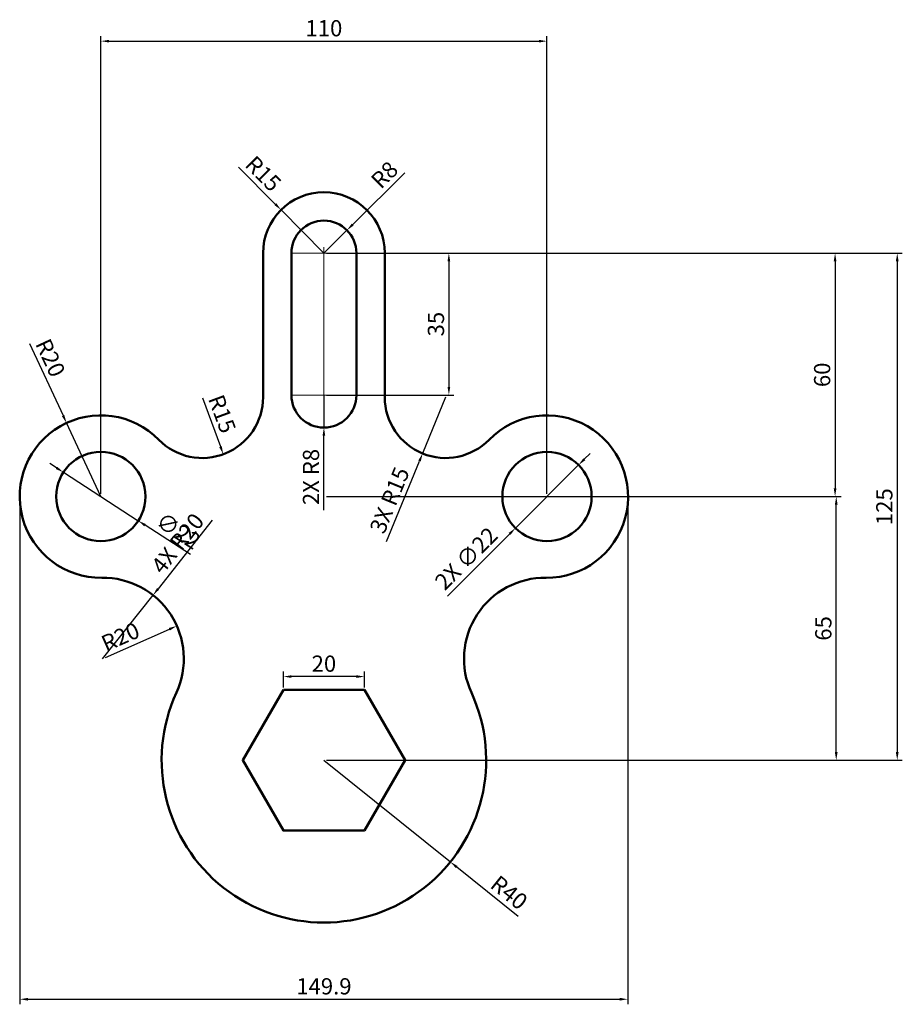
# Model space of a CAD drawing. Units: millimetres. Extents: x -2 to 216, y -10 to 233.
import ezdxf

# ---------------------------------------------------------------- set-up
doc = ezdxf.new("R2010")
doc.units = ezdxf.units.MM
doc.linetypes.add('CENTER', pattern=[50.8, 31.75, -6.35, 6.35, -6.35])
for name, color, linetype, lineweight in [('M-CNTR', 4, 'CENTER', 18), ('M-DIMS', 2, 'Continuous', 25), ('M-OUTL', 7, 'Continuous', 50)]:
    doc.layers.add(name, color=color, linetype=linetype, lineweight=lineweight)
doc.styles.get("Standard").update_dxf_attribs({"font": 'arial.ttf'})
doc.dimstyles.new('ISO-25', dxfattribs={"dimtxt": 4, "dimasz": 2, "dimexe": 1.25, "dimexo": 0.625, "dimtad": 1, "dimtxsty": 'Standard', "dimcen": 2.5, "dimadec": 0, "dimazin": 0, "dimtfac": 1, "dimtmove": 0, "dimatfit": 3, "dimfxl": 1, "dimarcsym": 0})

# ---------------------------------------------------------------- blocks, each defined once
blk = doc.blocks.new('*D1')
at = {"layer": 'Defpoints', "color": 0, "transparency": 16777216}
for p in [(128.44, 227.77), (18.44, 115.53), (128.44, 115.53)]:
    blk.add_point(p, dxfattribs=at)
at = {"layer": 'M-DIMS', "color": 0, "lineweight": -2, "transparency": 16777216}
for p, q in [((18.44, 116.16), (18.44, 229.02)), ((128.44, 116.16), (128.44, 229.02)), ((20.44, 227.77), (126.44, 227.77))]:
    blk.add_line(p, q, dxfattribs=at)
at = {"layer": 'M-DIMS', "color": 0, "transparency": 16777216}
for points in [[(20.44, 228.1), (20.44, 227.44), (18.44, 227.77)], [(126.44, 228.1), (126.44, 227.44), (128.44, 227.77)]]:
    blk.add_solid(points, dxfattribs=at)
at = {"layer": 'M-DIMS', "color": 0, "transparency": 16777216, "insert": (73.44, 230.44), "char_height": 4, "attachment_point": 5}
blk.add_mtext('110', dxfattribs=at)
blk = doc.blocks.new('*D2')
at = {"layer": 'Defpoints', "color": 0, "transparency": 16777216}
for p in [(73.44, 175.53), (73.44, 140.53), (104.25, 140.53)]:
    blk.add_point(p, dxfattribs=at)
at = {"layer": 'M-DIMS', "color": 0, "lineweight": -2, "transparency": 16777216}
for p, q in [((74.06, 175.53), (105.5, 175.53)), ((104.25, 173.53), (104.25, 142.53)), ((74.06, 140.53), (105.5, 140.53))]:
    blk.add_line(p, q, dxfattribs=at)
at = {"layer": 'M-DIMS', "color": 0, "transparency": 16777216}
for points in [[(103.92, 173.53), (104.58, 173.53), (104.25, 175.53)], [(103.92, 142.53), (104.58, 142.53), (104.25, 140.53)]]:
    blk.add_solid(points, dxfattribs=at)
at = {"layer": 'M-DIMS', "color": 0, "transparency": 16777216, "insert": (101.58, 158.03), "char_height": 4, "attachment_point": 5, "rotation": 90}
blk.add_mtext('35', dxfattribs=at)
blk = doc.blocks.new('*D3')
at = {"layer": 'Defpoints', "color": 0, "transparency": 16777216}
for p in [(63.44, 71.16), (63.44, 67.86), (83.44, 67.86)]:
    blk.add_point(p, dxfattribs=at)
at = {"layer": 'M-DIMS', "color": 0, "lineweight": -2, "transparency": 16777216}
for p, q in [((63.44, 68.48), (63.44, 72.41)), ((81.44, 71.16), (65.44, 71.16)), ((83.44, 68.48), (83.44, 72.41))]:
    blk.add_line(p, q, dxfattribs=at)
at = {"layer": 'M-DIMS', "color": 0, "transparency": 16777216}
for points in [[(65.44, 71.49), (65.44, 70.83), (63.44, 71.16)], [(81.44, 71.49), (81.44, 70.83), (83.44, 71.16)]]:
    blk.add_solid(points, dxfattribs=at)
at = {"layer": 'M-DIMS', "color": 0, "transparency": 16777216, "insert": (73.44, 73.83), "char_height": 4, "attachment_point": 5}
blk.add_mtext('20', dxfattribs=at)
blk = doc.blocks.new('*D4')
at = {"layer": 'Defpoints', "color": 0, "transparency": 16777216}
for p in [(73.44, 50.53), (104.62, 25.48)]:
    blk.add_point(p, dxfattribs=at)
at = {"layer": 'M-DIMS', "color": 0, "lineweight": -2, "transparency": 16777216}
for p, q in [((73.44, 50.53), (104.62, 25.48)), ((121.31, 12.06), (106.18, 24.22))]:
    blk.add_line(p, q, dxfattribs=at)
at = {"layer": 'M-DIMS', "color": 0, "transparency": 16777216}
blk.add_solid([(106.38, 24.48), (105.97, 23.96), (104.62, 25.48)], dxfattribs=at)
at = {"layer": 'M-DIMS', "color": 0, "transparency": 16777216, "insert": (118.78, 17.52), "char_height": 4, "attachment_point": 5, "rotation": 321.2128}
blk.add_mtext('R40', dxfattribs=at)
blk = doc.blocks.new('*D5')
at = {"layer": 'Defpoints', "color": 0, "transparency": 16777216}
for p in [(37.18, 83.65), (18.89, 75.54)]:
    blk.add_point(p, dxfattribs=at)
at = {"layer": 'M-DIMS', "color": 0, "lineweight": -2, "transparency": 16777216}
blk.add_line((19.62, 75.86), (35.35, 82.84), dxfattribs=at)
at = {"layer": 'M-DIMS', "color": 0, "transparency": 16777216}
blk.add_solid([(35.21, 83.14), (35.48, 82.53), (37.18, 83.65)], dxfattribs=at)
at = {"layer": 'M-DIMS', "color": 0, "transparency": 16777216, "insert": (23.47, 80.49), "char_height": 4, "attachment_point": 5, "rotation": 23.9265}
blk.add_mtext('R20', dxfattribs=at)
blk = doc.blocks.new('*D6')
at = {"layer": 'Defpoints', "color": 0, "transparency": 16777216}
for p in [(73.44, 115.53), (199.75, 115.53), (73.44, 50.53)]:
    blk.add_point(p, dxfattribs=at)
at = {"layer": 'M-DIMS', "color": 0, "lineweight": -2, "transparency": 16777216}
for p, q in [((74.06, 115.53), (201, 115.53)), ((199.75, 52.53), (199.75, 113.53)), ((74.06, 50.53), (201, 50.53))]:
    blk.add_line(p, q, dxfattribs=at)
at = {"layer": 'M-DIMS', "color": 0, "transparency": 16777216}
for points in [[(199.41, 113.53), (200.08, 113.53), (199.75, 115.53)], [(199.41, 52.53), (200.08, 52.53), (199.75, 50.53)]]:
    blk.add_solid(points, dxfattribs=at)
at = {"layer": 'M-DIMS', "color": 0, "transparency": 16777216, "insert": (197.08, 83.03), "char_height": 4, "attachment_point": 5, "rotation": 90}
blk.add_mtext('65', dxfattribs=at)
blk = doc.blocks.new('*D7')
at = {"layer": 'Defpoints', "color": 0, "transparency": 16777216}
for p in [(73.44, 175.53), (73.44, 115.53), (199.46, 115.53)]:
    blk.add_point(p, dxfattribs=at)
at = {"layer": 'M-DIMS', "color": 0, "lineweight": -2, "transparency": 16777216}
for p, q in [((74.06, 175.53), (200.71, 175.53)), ((199.46, 173.53), (199.46, 117.53)), ((74.06, 115.53), (200.71, 115.53))]:
    blk.add_line(p, q, dxfattribs=at)
at = {"layer": 'M-DIMS', "color": 0, "transparency": 16777216}
for points in [[(199.13, 173.53), (199.79, 173.53), (199.46, 175.53)], [(199.13, 117.53), (199.79, 117.53), (199.46, 115.53)]]:
    blk.add_solid(points, dxfattribs=at)
at = {"layer": 'M-DIMS', "color": 0, "transparency": 16777216, "insert": (196.79, 145.53), "char_height": 4, "attachment_point": 5, "rotation": 90}
blk.add_mtext('60', dxfattribs=at)
blk = doc.blocks.new('*D8')
at = {"layer": 'Defpoints', "color": 0, "transparency": 16777216}
for p in [(73.44, 175.53), (73.44, 50.53), (214.79, 50.53)]:
    blk.add_point(p, dxfattribs=at)
at = {"layer": 'M-DIMS', "color": 0, "lineweight": -2, "transparency": 16777216}
for p, q in [((74.06, 175.53), (216.04, 175.53)), ((214.79, 173.53), (214.79, 52.53)), ((74.06, 50.53), (216.04, 50.53))]:
    blk.add_line(p, q, dxfattribs=at)
at = {"layer": 'M-DIMS', "color": 0, "transparency": 16777216}
for points in [[(214.45, 173.53), (215.12, 173.53), (214.79, 175.53)], [(214.45, 52.53), (215.12, 52.53), (214.79, 50.53)]]:
    blk.add_solid(points, dxfattribs=at)
at = {"layer": 'M-DIMS', "color": 0, "transparency": 16777216, "insert": (212.12, 113.03), "char_height": 4, "attachment_point": 5, "rotation": 90}
blk.add_mtext('125', dxfattribs=at)
blk = doc.blocks.new('*D9')
at = {"layer": 'Defpoints', "color": 0, "transparency": 16777216}
for p in [(79.12, 181.17), (73.44, 175.53)]:
    blk.add_point(p, dxfattribs=at)
at = {"layer": 'M-DIMS', "color": 0, "lineweight": -2, "transparency": 16777216}
for p, q in [((93.36, 195.28), (80.54, 182.58)), ((73.44, 175.53), (79.12, 181.17))]:
    blk.add_line(p, q, dxfattribs=at)
at = {"layer": 'M-DIMS', "color": 0, "transparency": 16777216}
blk.add_solid([(80.3, 182.81), (80.77, 182.34), (79.12, 181.17)], dxfattribs=at)
at = {"layer": 'M-DIMS', "color": 0, "transparency": 16777216, "insert": (88.74, 194.46), "char_height": 4, "attachment_point": 5, "rotation": 44.7539}
blk.add_mtext('R8', dxfattribs=at)
blk = doc.blocks.new('*D10')
at = {"layer": 'Defpoints', "color": 0, "transparency": 16777216}
for p in [(62.87, 186.18), (73.44, 175.53)]:
    blk.add_point(p, dxfattribs=at)
at = {"layer": 'M-DIMS', "color": 0, "lineweight": -2, "transparency": 16777216}
for p, q in [((52.42, 196.72), (61.46, 187.6)), ((73.44, 175.53), (62.87, 186.18))]:
    blk.add_line(p, q, dxfattribs=at)
at = {"layer": 'M-DIMS', "color": 0, "transparency": 16777216}
blk.add_solid([(61.7, 187.84), (61.23, 187.37), (62.87, 186.18)], dxfattribs=at)
at = {"layer": 'M-DIMS', "color": 0, "transparency": 16777216, "insert": (58.13, 194.75), "char_height": 4, "attachment_point": 5, "rotation": 314.776}
blk.add_mtext('R15', dxfattribs=at)
blk = doc.blocks.new('*D11')
at = {"layer": 'Defpoints', "color": 0, "transparency": 16777216}
for p in [(43.44, 140.03), (48.63, 125.96)]:
    blk.add_point(p, dxfattribs=at)
at = {"layer": 'M-DIMS', "color": 0, "lineweight": -2, "transparency": 16777216}
blk.add_line((43.49, 139.88), (47.93, 127.83), dxfattribs=at)
at = {"layer": 'M-DIMS', "color": 0, "transparency": 16777216}
blk.add_solid([(48.25, 127.95), (47.62, 127.72), (48.63, 125.96)], dxfattribs=at)
at = {"layer": 'M-DIMS', "color": 0, "transparency": 16777216, "insert": (47.87, 135.72), "char_height": 4, "attachment_point": 5, "rotation": 290.2358}
blk.add_mtext('R15', dxfattribs=at)
blk = doc.blocks.new('*D12')
at = {"layer": 'Defpoints', "color": 0, "transparency": 16777216}
for p in [(9.2, 121.51), (27.67, 109.56)]:
    blk.add_point(p, dxfattribs=at)
at = {"layer": 'M-DIMS', "color": 0, "lineweight": -2, "transparency": 16777216}
for p, q in [((7.52, 122.6), (5.84, 123.68)), ((9.2, 121.51), (27.67, 109.56)), ((40.51, 101.25), (29.35, 108.47))]:
    blk.add_line(p, q, dxfattribs=at)
at = {"layer": 'M-DIMS', "color": 0, "transparency": 16777216}
for points in [[(7.7, 122.88), (7.34, 122.32), (9.2, 121.51)], [(29.53, 108.75), (29.17, 108.19), (27.67, 109.56)]]:
    blk.add_solid(points, dxfattribs=at)
at = {"layer": 'M-DIMS', "color": 0, "transparency": 16777216, "insert": (37.28, 106.65), "char_height": 4, "attachment_point": 5, "rotation": 327.0916}
blk.add_mtext('∅22', dxfattribs=at)
blk = doc.blocks.new('*D13')
at = {"layer": 'Defpoints', "color": 0, "transparency": 16777216}
for p in [(9.99, 133.66), (18.44, 115.53)]:
    blk.add_point(p, dxfattribs=at)
at = {"layer": 'M-DIMS', "color": 0, "lineweight": -2, "transparency": 16777216}
for p, q in [((0.85, 153.26), (9.14, 135.47)), ((18.44, 115.53), (9.99, 133.66))]:
    blk.add_line(p, q, dxfattribs=at)
at = {"layer": 'M-DIMS', "color": 0, "transparency": 16777216}
blk.add_solid([(9.44, 135.62), (8.84, 135.33), (9.99, 133.66)], dxfattribs=at)
at = {"layer": 'M-DIMS', "color": 0, "transparency": 16777216, "insert": (5.55, 149.5), "char_height": 4, "attachment_point": 5, "rotation": 294.9922}
blk.add_mtext('R20', dxfattribs=at)
blk = doc.blocks.new('MOUNT-HOLE-D22')
blk.add_circle((11, 11), 11)
blk = doc.blocks.new('*D15')
at = {"layer": 'Defpoints', "color": 0, "transparency": 16777216}
for p in [(-1.52, 116.88), (148.39, 116.88), (148.39, -8.37)]:
    blk.add_point(p, dxfattribs=at)
at = {"layer": 'M-DIMS', "color": 0, "lineweight": -2, "transparency": 16777216}
for p, q in [((-1.52, 116.25), (-1.52, -9.62)), ((148.39, 116.25), (148.39, -9.62)), ((0.48, -8.37), (146.39, -8.37))]:
    blk.add_line(p, q, dxfattribs=at)
at = {"layer": 'M-DIMS', "color": 0, "transparency": 16777216}
for points in [[(0.48, -8.03), (0.48, -8.7), (-1.52, -8.37)], [(146.39, -8.03), (146.39, -8.7), (148.39, -8.37)]]:
    blk.add_solid(points, dxfattribs=at)
at = {"layer": 'M-DIMS', "color": 0, "transparency": 16777216, "insert": (73.44, -5.7), "char_height": 4, "attachment_point": 5}
blk.add_mtext('149.9', dxfattribs=at)
blk = doc.blocks.new('*D16')
at = {"layer": 'Defpoints', "color": 0, "transparency": 16777216}
for p in [(136.22, 123.31), (120.66, 107.76)]:
    blk.add_point(p, dxfattribs=at)
at = {"layer": 'M-DIMS', "color": 0, "lineweight": -2, "transparency": 16777216}
for p, q in [((137.63, 124.73), (139.05, 126.14)), ((136.22, 123.31), (120.66, 107.76)), ((103.87, 90.97), (119.24, 106.34))]:
    blk.add_line(p, q, dxfattribs=at)
at = {"layer": 'M-DIMS', "color": 0, "transparency": 16777216}
for points in [[(137.4, 124.96), (137.87, 124.49), (136.22, 123.31)], [(119.01, 106.58), (119.48, 106.11), (120.66, 107.76)]]:
    blk.add_solid(points, dxfattribs=at)
at = {"layer": 'M-DIMS', "color": 0, "transparency": 16777216, "insert": (108.88, 99.92), "char_height": 4, "attachment_point": 5, "rotation": 44.9914}
blk.add_mtext('2X ∅22', dxfattribs=at)
blk = doc.blocks.new('*D17')
at = {"layer": 'Defpoints', "color": 0, "transparency": 16777216}
for p in [(103.44, 140.03), (97.77, 126.14)]:
    blk.add_point(p, dxfattribs=at)
at = {"layer": 'M-DIMS', "color": 0, "lineweight": -2, "transparency": 16777216}
for p, q in [((103.44, 140.03), (97.77, 126.14)), ((88.91, 104.45), (97.01, 124.29))]:
    blk.add_line(p, q, dxfattribs=at)
at = {"layer": 'M-DIMS', "color": 0, "transparency": 16777216}
blk.add_solid([(96.7, 124.42), (97.32, 124.16), (97.77, 126.14)], dxfattribs=at)
at = {"layer": 'M-DIMS', "color": 0, "transparency": 16777216, "insert": (90.11, 114.45), "char_height": 4, "attachment_point": 5, "rotation": 67.794}
blk.add_mtext('3X R15', dxfattribs=at)
blk = doc.blocks.new('*D18')
at = {"layer": 'Defpoints', "color": 0, "transparency": 16777216}
for p in [(31.31, 91.22), (18.89, 75.54)]:
    blk.add_point(p, dxfattribs=at)
at = {"layer": 'M-DIMS', "color": 0, "lineweight": -2, "transparency": 16777216}
for p, q in [((45.93, 109.68), (32.55, 92.78)), ((18.89, 75.54), (31.31, 91.22))]:
    blk.add_line(p, q, dxfattribs=at)
at = {"layer": 'M-DIMS', "color": 0, "transparency": 16777216}
blk.add_solid([(32.29, 92.99), (32.82, 92.58), (31.31, 91.22)], dxfattribs=at)
at = {"layer": 'M-DIMS', "color": 0, "transparency": 16777216, "insert": (37.77, 103.67), "char_height": 4, "attachment_point": 5, "rotation": 51.6198}
blk.add_mtext('4X R20', dxfattribs=at)
blk = doc.blocks.new('*D19')
at = {"layer": 'Defpoints', "color": 0, "transparency": 16777216}
for p in [(73.44, 140.53), (73.44, 132.53)]:
    blk.add_point(p, dxfattribs=at)
at = {"layer": 'M-DIMS', "color": 0, "lineweight": -2, "transparency": 16777216}
for p, q in [((73.44, 140.53), (73.44, 132.53)), ((73.44, 112.16), (73.44, 130.53))]:
    blk.add_line(p, q, dxfattribs=at)
at = {"layer": 'M-DIMS', "color": 0, "transparency": 16777216}
blk.add_solid([(73.1, 130.53), (73.77, 130.53), (73.44, 132.53)], dxfattribs=at)
at = {"layer": 'M-DIMS', "color": 0, "transparency": 16777216, "insert": (70.77, 120.35), "char_height": 4, "attachment_point": 5, "rotation": 89.9986}
blk.add_mtext('2X R8', dxfattribs=at)

msp = doc.modelspace()

# ---------------------------------------------------------------- linework, layer by layer
at = {"layer": 'M-CNTR'}
for p, q in [((73.437, 132.535), (73.437, 183.535)), ((69.482, 175.535), (65.437, 175.535)), ((73.437, 175.535), (69.482, 175.535)), ((73.437, 132.535), (73.437, 175.535)), ((73.437, 175.535), (73.437, 140.535)), ((73.437, 175.535), (81.437, 175.535)), ((67.983, 140.535), (65.437, 140.535)), ((73.437, 140.535), (67.983, 140.535)), ((73.437, 140.535), (81.437, 140.535))]:
    msp.add_line(p, q, dxfattribs=at)
at = {"layer": 'M-OUTL'}
for p, q in [((58.437, 175.535), (58.437, 140.03)), ((65.437, 175.535), (65.437, 140.535)), ((81.437, 175.535), (81.437, 140.535)), ((88.437, 175.535), (88.437, 140.03))]:
    msp.add_line(p, q, dxfattribs=at)
msp.add_lwpolyline([(63.437, 67.855), (53.437, 50.535), (63.437, 33.214), (83.437, 33.214), (93.437, 50.535), (83.437, 67.855)], close=True, dxfattribs=at)
for centre, radius, start, end in [((73.437, 175.535), 15, 0, 180), ((73.437, 175.535), 8, 0, 180), ((43.437, 140.03), 15, 224.41531, 0), ((73.437, 140.535), 8, 180, 0), ((103.437, 140.03), 15, 180, 315.58469), ((18.437, 115.535), 20, 44.41531, 270.65553), ((128.437, 115.535), 20, 269.34447, 135.58469), ((18.895, 75.537), 20, 335.37293, 90.65553), ((127.98, 75.537), 20, 89.34447, 204.62707), ((73.437, 50.535), 40, 155.37293, 24.62707)]:
    msp.add_arc(centre, radius, start, end, dxfattribs=at)

# ---------------------------------------------------------------- block references
for p in [(7.437, 104.535), (117.437, 104.535)]:
    msp.add_blockref('MOUNT-HOLE-D22', p, dxfattribs=at)

# ---------------------------------------------------------------- dimensions: what is measured, and where the dimension line sits
at = {"layer": 'M-DIMS'}
for base, p1, p2, override, picture, middle in [((128.437, 227.77), (18.437, 115.535), (128.437, 115.535), {"dimclrd": 0, "dimclre": 0, "dimclrt": 0}, '*D1', (73.437, 230.437)), ((148.394, -8.365), (-1.519, 116.879), (148.394, 116.879), {"dimdec": 1, "dimlfac": 1, "dimrnd": 0, "dimzin": 0, "dimdsep": 46, "dimlunit": 2}, '*D15', (73.437, -5.698)), ((63.437, 71.16), (83.437, 67.855), (63.437, 67.855), {"dimclrd": 0, "dimclre": 0, "dimclrt": 0}, '*D3', (73.437, 73.827))]:
    dim = msp.add_linear_dim(base=base, p1=p1, p2=p2, dimstyle='ISO-25', override=override, dxfattribs=at)
    dim.commit()
    dim.dimension.update_dxf_attribs({"geometry": picture, "text_midpoint": middle})
dim = msp.add_radius_dim(center=(73.437, 175.535), mpoint=(62.872, 186.183), dimstyle='ISO-25', override={"dimclrd": 0, "dimclre": 0, "dimclrt": 0}, dxfattribs=at)
dim.commit()
dim.dimension.update_dxf_attribs({"geometry": '*D10', "text_midpoint": (58.131, 194.748)})
for center, mpoint, picture, middle in [((73.437, 175.535), (79.118, 181.167), '*D9', (90.62, 192.571)), ((18.437, 115.535), (9.987, 133.662), '*D13', (3.131, 148.37)), ((43.437, 140.03), (48.625, 125.956), '*D11', (45.368, 134.793)), ((18.895, 75.537), (37.176, 83.649), '*D5', (24.555, 78.049)), ((73.437, 50.535), (104.616, 25.478), '*D4', (117.106, 15.441))]:
    dim = msp.add_radius_dim(center=center, mpoint=mpoint, dimstyle='ISO-25', override={"dimclrd": 0, "dimclre": 0, "dimclrt": 0}, dxfattribs=at)
    dim.commit()
    dim.dimension.update_dxf_attribs({"geometry": picture, "text_midpoint": middle, "dimtype": 164})
for base, p1, p2, picture, middle in [((104.251, 140.535), (73.437, 175.535), (73.437, 140.535), '*D2', (101.582, 158.035)), ((199.461, 115.535), (73.437, 175.535), (73.437, 115.535), '*D7', (196.793, 145.535)), ((214.788, 50.535), (73.437, 175.535), (73.437, 50.535), '*D8', (212.121, 113.035)), ((199.747, 115.535), (73.437, 50.535), (73.437, 115.535), '*D6', (197.08, 83.035))]:
    dim = msp.add_linear_dim(base=base, p1=p1, p2=p2, angle=90, dimstyle='ISO-25', override={"dimclrd": 0, "dimclre": 0, "dimclrt": 0}, dxfattribs=at)
    dim.commit()
    dim.dimension.update_dxf_attribs({"geometry": picture, "text_midpoint": middle})
for center, mpoint, text, picture, middle in [((73.437, 140.535), (73.437, 132.535), '2X <>', '*D19', (70.769, 120.349)), ((103.437, 140.03), (97.768, 126.142), '3X <>', '*D17', (90.114, 114.453)), ((18.895, 75.537), (31.312, 91.216), '4X <>', '*D18', (37.774, 103.67))]:
    dim = msp.add_radius_dim(center=center, mpoint=mpoint, text=text, dimstyle='ISO-25', override={"dimdec": 0, "dimlfac": 1, "dimrnd": 0, "dimzin": 0, "dimdsep": 46, "dimlunit": 2}, dxfattribs=at)
    dim.commit()
    dim.dimension.update_dxf_attribs({"geometry": picture, "text_midpoint": middle})
dim = msp.add_diameter_dim_2p(p1=(136.217, 123.312), p2=(120.658, 107.758), text='2X <>', dimstyle='ISO-25', override={"dimdec": 0, "dimlfac": 1, "dimrnd": 0, "dimzin": 0, "dimdsep": 46, "dimlunit": 2}, dxfattribs=at)
dim.commit()
dim.dimension.update_dxf_attribs({"geometry": '*D16', "text_midpoint": (110.848, 97.951)})
dim = msp.add_diameter_dim_2p(p1=(9.202, 121.511), p2=(27.672, 109.559), dimstyle='ISO-25', override={"dimclrd": 0, "dimclre": 0, "dimclrt": 0}, dxfattribs=at)
dim.commit()
dim.dimension.update_dxf_attribs({"geometry": '*D12', "text_midpoint": (35.77, 104.318), "dimtype": 163})

doc.saveas('drawing.dxf')
